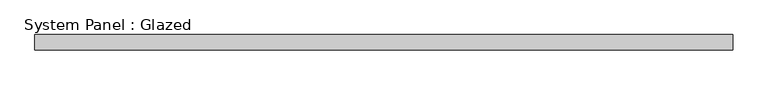
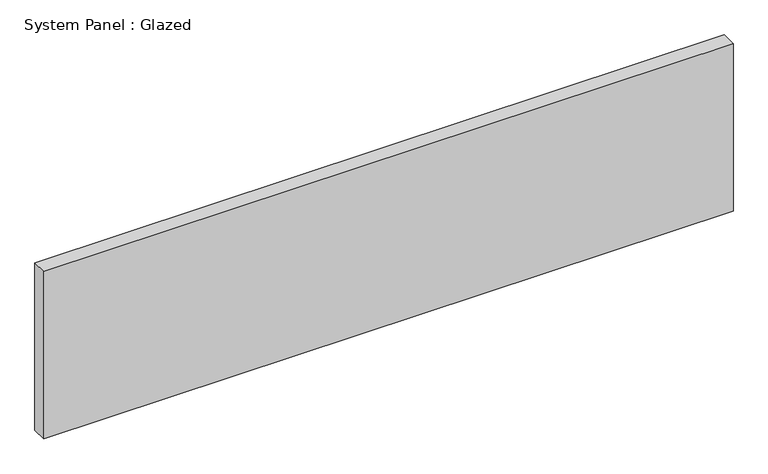
"""IFC4 building model written with IfcOpenShell, lengths in millimetres: plate geometry, System Panel : Glazed."""

from ifc_helpers import new_model, si_unit, origin, origin_with_axes, place, context, project, spatial, polyline, outline, extrude, source, transform, mapped, element, save


def system_panel_glazed_14aec0f7(model_context):
    return source(origin(), model_context, "Body", "SweptSolid", [
        extrude(outline(polyline([(572.42075, 19.05), (-572.42075, 19.05), (-572.42075, 44.45), (572.42075, 44.45), (572.42075, 19.05)])), origin_with_axes(), (0.0, 0.0, 1.0), 293.9415),
    ])


if __name__ == "__main__":
    model = new_model("IFC4")
    model_context = context("Model", 3, world=origin())
    ifc_project = project(units=[si_unit("LENGTHUNIT", "METRE", prefix="MILLI")], contexts=[model_context])
    site = spatial("IfcSite", under=ifc_project)
    building = spatial("IfcBuilding", under=site)
    placement = place(None, origin())
    system_panel_glazed_shape = system_panel_glazed_14aec0f7(model_context)
    element("IfcPlate", 1, ObjectType="System Panel : Glazed", at=placement, inside=building, context=model_context, shape_type="MappedRepresentation", body=[
        mapped(system_panel_glazed_shape, transform((0.0, 0.0, 0.0), x_axis=(1.0, 0.0, 0.0), y_axis=(0.0, 1.0, 0.0), z_axis=(0.0, 0.0, 1.0))),
    ])
    save(model, "model.ifc")

# Revit data of these elements
# Type "System Panel : Glazed"
#   Construction Type Id = "GSP4R"
#   Analytic Construction = "1/8 in Pilkington single glazing"
#   Visual Light Transmittance = 0.9
#   Solar Heat Gain Coefficient = 0.86
#   Heat Transfer Coefficient (U) = 1.18115 BTU/(h·ft²·°F)
#   Define Thermal Properties by = 1
# Element 1 (IfcPlate, "System Panel : Glazed")
#   Materials on its faces: "Glass"
# Materials
#   "Glass": class "Glass", colour RGB 0 128 192, transparency 0.75, Description = "Soda Lime Glass", Cost = 0
